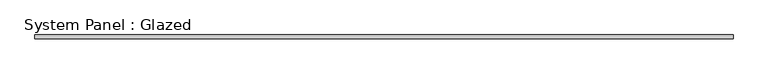
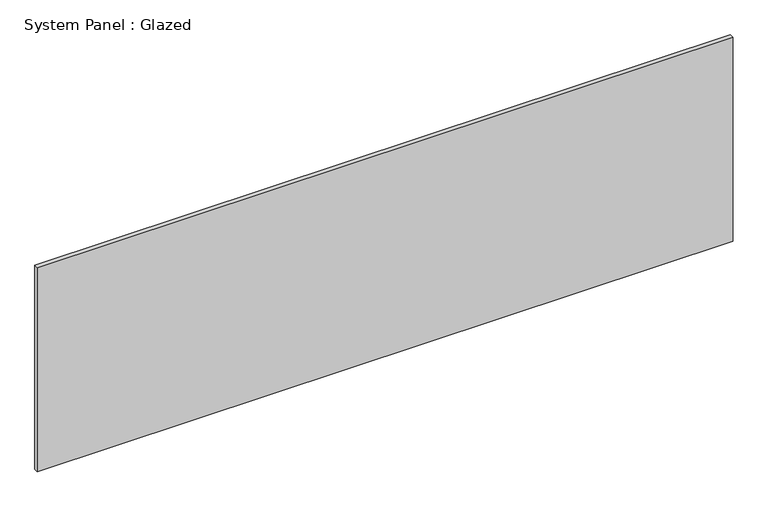
"""IFC4 building model written with IfcOpenShell, lengths in millimetres: plate geometry, System Panel : Glazed."""

from ifc_helpers import new_model, si_unit, origin, origin_with_axes, place, context, project, spatial, polyline, outline, extrude, source, transform, mapped, element, save


def system_panel_glazed_7dd8e57f(model_context):
    return source(origin(), model_context, "Body", "SweptSolid", [
        extrude(outline(polyline([(2355.85, 19.05), (-2355.85, 19.05), (-2355.85, 44.45), (2355.85, 44.45), (2355.85, 19.05)])), origin_with_axes(), (0.0, 0.0, 1.0), 1460.5),
    ])


if __name__ == "__main__":
    model = new_model("IFC4")
    model_context = context("Model", 3, world=origin())
    ifc_project = project(units=[si_unit("LENGTHUNIT", "METRE", prefix="MILLI")], contexts=[model_context])
    site = spatial("IfcSite", under=ifc_project)
    building = spatial("IfcBuilding", under=site)
    placement = place(None, origin())
    system_panel_glazed_shape = system_panel_glazed_7dd8e57f(model_context)
    element("IfcPlate", 1, ObjectType="System Panel : Glazed", at=placement, inside=building, context=model_context, shape_type="MappedRepresentation", body=[
        mapped(system_panel_glazed_shape, transform((0.0, 0.0, 0.0), x_axis=(1.0, 0.0, 0.0), y_axis=(0.0, 1.0, 0.0), z_axis=(0.0, 0.0, 1.0))),
    ])
    save(model, "model.ifc")

# Revit data of these elements
# Type "System Panel : Glazed"
#   Construction Type Id = "GSP4R"
#   Analytic Construction = "1/8 in Pilkington single glazing"
#   Visual Light Transmittance = 0.9
#   Solar Heat Gain Coefficient = 0.86
#   Heat Transfer Coefficient (U) = 1.18115 BTU/(h·ft²·°F)
# Element 1 (IfcPlate, "System Panel : Glazed")
#   Materials on its faces: "Glass"
# Materials
#   "Glass": class "Glass", colour RGB 0 128 192, transparency 0.75, Description = "Soda Lime Glass", Cost = 0
